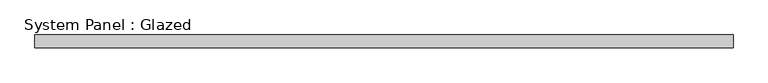
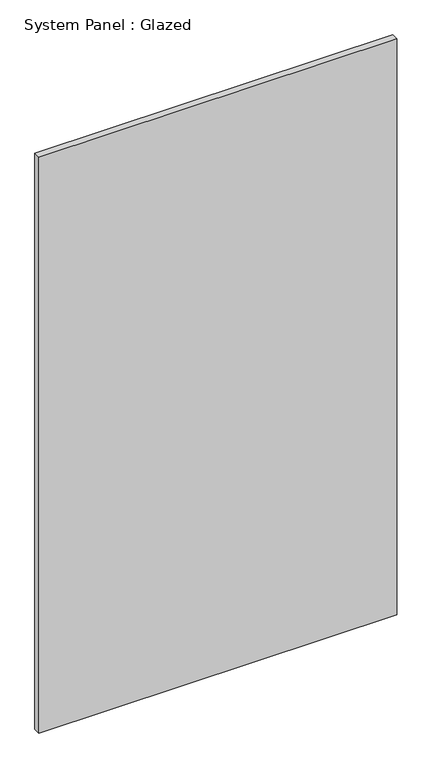
"""IFC4 building model written with IfcOpenShell, lengths in millimetres: plate geometry, System Panel : Glazed."""

from ifc_helpers import new_model, si_unit, origin, origin_with_axes, place, context, project, spatial, polyline, outline, extrude, source, transform, mapped, element, save


def system_panel_glazed_7e177a0b(model_context):
    return source(origin(), model_context, "Body", "SweptSolid", [
        extrude(outline(polyline([(688.9750001, 19.05), (-688.9750001, 19.05), (-688.9750001, 44.45), (688.9750001, 44.45), (688.9750001, 19.05)])), origin_with_axes(), (0.0, 0.0, 1.0), 2343.15),
    ])


if __name__ == "__main__":
    model = new_model("IFC4")
    model_context = context("Model", 3, world=origin())
    ifc_project = project(units=[si_unit("LENGTHUNIT", "METRE", prefix="MILLI")], contexts=[model_context])
    site = spatial("IfcSite", under=ifc_project)
    building = spatial("IfcBuilding", under=site)
    placement = place(None, origin())
    system_panel_glazed_shape = system_panel_glazed_7e177a0b(model_context)
    element("IfcPlate", 1, ObjectType="System Panel : Glazed", at=placement, inside=building, context=model_context, shape_type="MappedRepresentation", body=[
        mapped(system_panel_glazed_shape, transform((0.0, 0.0, 0.0), x_axis=(1.0, 0.0, 0.0), y_axis=(0.0, 1.0, 0.0), z_axis=(0.0, 0.0, 1.0))),
    ])
    save(model, "model.ifc")

# Revit data of these elements
# Type "System Panel : Glazed"
#   Construction Type Id = "GSP4R"
#   Analytic Construction = "1/8 in Pilkington single glazing"
#   Visual Light Transmittance = 0.9
#   Solar Heat Gain Coefficient = 0.86
#   Heat Transfer Coefficient (U) = 1.18115 BTU/(h·ft²·°F)
#   Define Thermal Properties by = 1
# Element 1 (IfcPlate, "System Panel : Glazed")
#   Materials on its faces: "Glass"
# Materials
#   "Glass": class "Glass", colour RGB 0 128 192, transparency 0.75, Description = "Soda Lime Glass", Cost = 0
